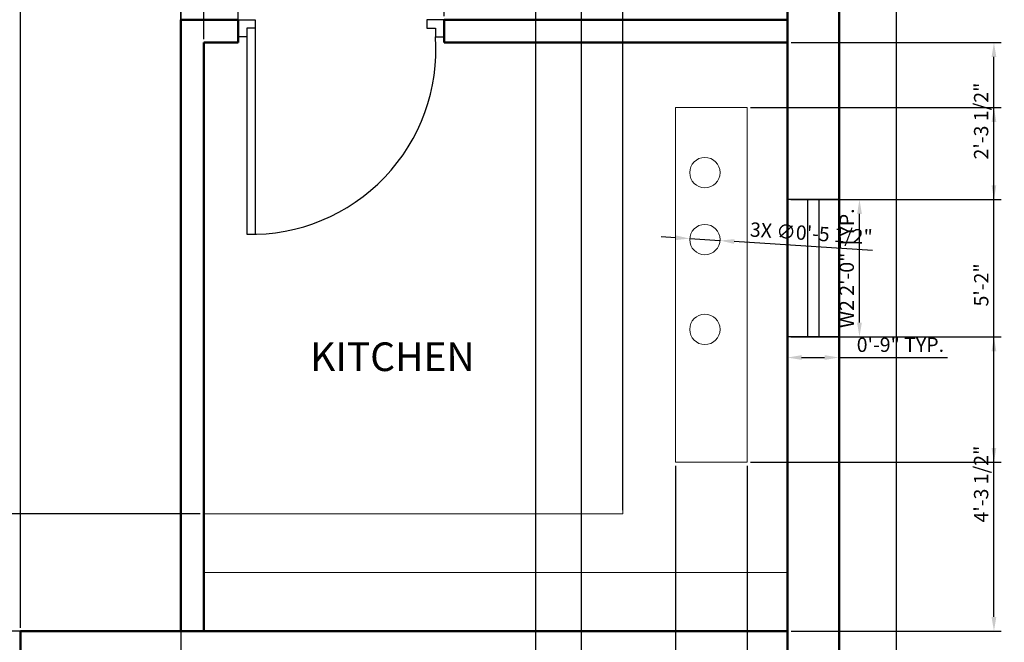
# Model space of a CAD drawing. Units: inches. Extents: x 1905 to 2315, y 3232 to 3824.
# Tile 4 of 8: x 2143 to 2315, y 3371 to 3479. Entities that reach past the tile are written whole.
import ezdxf

# ---------------------------------------------------------------- set-up
doc = ezdxf.new("R2010")
doc.units = ezdxf.units.IN
for name, color, linetype, lineweight in [('A-ANNO-DIMS', 2, 'Continuous', 18), ('A-AREA-IDEN', 7, 'Continuous', 25), ('A-EQPM', 9, 'Continuous', 18), ('A-FLOR-CABT', 8, 'Continuous', 18), ('door', 1, 'Continuous', 25), ('wall', 2, 'Continuous', 50), ('WINDOW', 60, 'Continuous', 25)]:
    doc.layers.add(name, color=color, linetype=linetype, lineweight=lineweight)
doc.styles.get("Standard").update_dxf_attribs({"font": 'arial.ttf'})
doc.dimstyles.new('ISO-25', dxfattribs={"dimtxt": 2.5, "dimasz": 2.5, "dimexe": 1.25, "dimexo": 0.625, "dimtad": 1, "dimdec": 1, "dimlunit": 3, "dimtxsty": 'Standard', "dimcen": 2.5, "dimadec": 0, "dimazin": 0, "dimtfac": 1, "dimtdec": 1, "dimtmove": 0, "dimatfit": 3, "dimfxl": 1, "dimarcsym": 0})

# ---------------------------------------------------------------- blocks, each defined once
blk = doc.blocks.new('*D16')
at = {"layer": 'A-ANNO-DIMS', "color": 0, "lineweight": -2, "transparency": 16777216}
for p, q in [((2286.63, 3793.23), (2297.23, 3793.23)), ((2295.98, 3790.73), (2295.98, 3279.73)), ((2286.63, 3277.23), (2297.23, 3277.23))]:
    blk.add_line(p, q, dxfattribs=at)
at = {"layer": 'A-ANNO-DIMS', "color": 0, "transparency": 16777216}
for points in [[(2295.57, 3790.73), (2296.4, 3790.73), (2295.98, 3793.23)], [(2295.57, 3279.73), (2296.4, 3279.73), (2295.98, 3277.23)]]:
    blk.add_solid(points, dxfattribs=at)
at = {"layer": 'Defpoints', "color": 0, "transparency": 16777216}
for p in [(2286.01, 3793.23), (2286.01, 3277.23), (2295.98, 3277.23)]:
    blk.add_point(p, dxfattribs=at)
at = {"layer": 'A-ANNO-DIMS', "color": 0, "transparency": 16777216, "insert": (2294.08, 3535.23), "char_height": 2.5, "attachment_point": 5, "rotation": 90}
blk.add_mtext("43'", dxfattribs=at)
blk = doc.blocks.new('DOOR-SWING-36IN')
for p, q in [((36.01, 34.5), (0.01, 34.5)), ((34.51, 36), (37.51, 36)), ((34.51, 34.5), (34.51, 36)), ((36.01, 34.5), (34.51, 34.5)), ((36.01, 33), (36.01, 34.5)), ((37.51, 36), (37.51, 33)), ((36.01, 33), (0.01, 33)), ((37.51, 33), (36.01, 33)), ((37.51, 3), (36.01, 3)), ((36.01, 3), (36.01, 1.5)), ((37.51, 0), (37.51, 3)), ((36.01, 1.5), (34.51, 1.5)), ((34.51, 1.5), (34.51, 0)), ((34.51, 0), (37.51, 0))]:
    blk.add_line(p, q)
blk.add_arc((32.32, 33.75), 32.32, 178.6705, 273.8756)
blk = doc.blocks.new('WIN-24IN')
for p, q in [((9, 24), (0, 24)), ((0, 24), (0, 0)), ((3.5, 24), (3.5, 0)), ((5.5, 24), (5.5, 0)), ((9, 24), (9, 0)), ((9, 0), (0, 0))]:
    blk.add_line(p, q)
blk = doc.blocks.new('*D23')
at = {"layer": 'A-ANNO-DIMS', "color": 0, "lineweight": -2, "transparency": 16777216}
for p, q in [((2286.6, 3448.02), (2290.82, 3448.02)), ((2289.57, 3426.52), (2289.57, 3445.52)), ((2286.6, 3424.02), (2290.82, 3424.02))]:
    blk.add_line(p, q, dxfattribs=at)
at = {"layer": 'A-ANNO-DIMS', "color": 0, "transparency": 16777216}
for points in [[(2289.16, 3445.52), (2289.99, 3445.52), (2289.57, 3448.02)], [(2289.16, 3426.52), (2289.99, 3426.52), (2289.57, 3424.02)]]:
    blk.add_solid(points, dxfattribs=at)
at = {"layer": 'Defpoints', "color": 0, "transparency": 16777216}
for p in [(2285.97, 3448.02), (2289.57, 3448.02), (2285.97, 3424.02)]:
    blk.add_point(p, dxfattribs=at)
at = {"layer": 'A-ANNO-DIMS', "color": 0, "transparency": 16777216, "insert": (2287.67, 3436.02), "char_height": 2.5, "attachment_point": 5, "rotation": 90}
blk.add_mtext('W2 2\'-0" TYP.', dxfattribs=at)
blk = doc.blocks.new('*D24')
at = {"layer": 'A-ANNO-DIMS', "color": 0, "lineweight": -2, "transparency": 16777216}
for p, q in [((2276.97, 3423.4), (2276.97, 3419.17)), ((2285.97, 3423.4), (2285.97, 3419.17)), ((2279.47, 3420.42), (2283.47, 3420.42)), ((2285.97, 3420.42), (2304.96, 3420.42))]:
    blk.add_line(p, q, dxfattribs=at)
at = {"layer": 'A-ANNO-DIMS', "color": 0, "transparency": 16777216}
for points in [[(2279.47, 3420.84), (2279.47, 3420.01), (2276.97, 3420.42)], [(2283.47, 3420.84), (2283.47, 3420.01), (2285.97, 3420.42)]]:
    blk.add_solid(points, dxfattribs=at)
at = {"layer": 'Defpoints', "color": 0, "transparency": 16777216}
for p in [(2276.97, 3424.02), (2285.97, 3424.02), (2285.97, 3420.42)]:
    blk.add_point(p, dxfattribs=at)
at = {"layer": 'A-ANNO-DIMS', "color": 0, "transparency": 16777216, "insert": (2296.72, 3422.33), "char_height": 2.5, "attachment_point": 5}
blk.add_mtext('0\'-9" TYP.', dxfattribs=at)
blk = doc.blocks.new('*D41')
at = {"layer": 'A-ANNO-DIMS', "color": 0, "lineweight": -2, "transparency": 16777216}
for p, q in [((2095.01, 3663.61), (2095.01, 3232.16)), ((2171.01, 3663.61), (2171.01, 3232.16)), ((2097.51, 3233.41), (2168.51, 3233.41))]:
    blk.add_line(p, q, dxfattribs=at)
at = {"layer": 'A-ANNO-DIMS', "color": 0, "transparency": 16777216}
for points in [[(2097.51, 3233.83), (2097.51, 3233), (2095.01, 3233.41)], [(2168.51, 3233.83), (2168.51, 3233), (2171.01, 3233.41)]]:
    blk.add_solid(points, dxfattribs=at)
at = {"layer": 'Defpoints', "color": 0, "transparency": 16777216}
for p in [(2095.01, 3664.23), (2171.01, 3664.23), (2171.01, 3233.41)]:
    blk.add_point(p, dxfattribs=at)
at = {"layer": 'A-ANNO-DIMS', "color": 0, "transparency": 16777216, "insert": (2133.01, 3235.31), "char_height": 2.5, "attachment_point": 5}
blk.add_mtext('6\'-4"', dxfattribs=at)
blk = doc.blocks.new('*D51')
at = {"layer": 'A-ANNO-DIMS', "color": 0, "lineweight": -2, "transparency": 16777216}
for p, q in [((2277.6, 3424.02), (2314.32, 3424.02)), ((2313.07, 3375.1), (2313.07, 3421.52)), ((2277.63, 3372.6), (2314.32, 3372.6))]:
    blk.add_line(p, q, dxfattribs=at)
at = {"layer": 'A-ANNO-DIMS', "color": 0, "transparency": 16777216}
for points in [[(2312.65, 3421.52), (2313.48, 3421.52), (2313.07, 3424.02)], [(2312.65, 3375.1), (2313.48, 3375.1), (2313.07, 3372.6)]]:
    blk.add_solid(points, dxfattribs=at)
at = {"layer": 'Defpoints', "color": 0, "transparency": 16777216}
for p in [(2276.97, 3424.02), (2313.07, 3424.02), (2277.01, 3372.6)]:
    blk.add_point(p, dxfattribs=at)
at = {"layer": 'A-ANNO-DIMS', "color": 0, "transparency": 16777216, "insert": (2311.15, 3398.31), "char_height": 2.5, "attachment_point": 5, "rotation": 90}
blk.add_mtext('4\'-3 1/2"', dxfattribs=at)
blk = doc.blocks.new('*D52')
at = {"layer": 'A-ANNO-DIMS', "color": 0, "lineweight": -2, "transparency": 16777216}
for p, q in [((2277.63, 3475.45), (2314.32, 3475.45)), ((2313.07, 3450.52), (2313.07, 3472.95)), ((2277.6, 3448.02), (2314.32, 3448.02))]:
    blk.add_line(p, q, dxfattribs=at)
at = {"layer": 'A-ANNO-DIMS', "color": 0, "transparency": 16777216}
for points in [[(2312.65, 3472.95), (2313.48, 3472.95), (2313.07, 3475.45)], [(2312.65, 3450.52), (2313.48, 3450.52), (2313.07, 3448.02)]]:
    blk.add_solid(points, dxfattribs=at)
at = {"layer": 'Defpoints', "color": 0, "transparency": 16777216}
for p in [(2277.01, 3475.45), (2313.07, 3475.45), (2276.97, 3448.02)]:
    blk.add_point(p, dxfattribs=at)
at = {"layer": 'A-ANNO-DIMS', "color": 0, "transparency": 16777216, "insert": (2311.15, 3461.74), "char_height": 2.5, "attachment_point": 5, "rotation": 90}
blk.add_mtext('2\'-3 1/2"', dxfattribs=at)
blk = doc.blocks.new('*D62')
at = {"layer": 'A-ANNO-DIMS', "color": 0, "lineweight": -2, "transparency": 16777216}
for p, q in [((2233.01, 3322.86), (2233.01, 3821.54)), ((2241.01, 3322.86), (2241.01, 3821.54)), ((2235.51, 3820.29), (2238.51, 3820.29))]:
    blk.add_line(p, q, dxfattribs=at)
at = {"layer": 'A-ANNO-DIMS', "color": 0, "transparency": 16777216}
for points in [[(2235.51, 3820.71), (2235.51, 3819.88), (2233.01, 3820.29)], [(2238.51, 3820.71), (2238.51, 3819.88), (2241.01, 3820.29)]]:
    blk.add_solid(points, dxfattribs=at)
at = {"layer": 'Defpoints', "color": 0, "transparency": 16777216}
for p in [(2241.01, 3820.29), (2233.01, 3322.23), (2241.01, 3322.23)]:
    blk.add_point(p, dxfattribs=at)
at = {"layer": 'A-ANNO-DIMS', "color": 0, "transparency": 16777216, "insert": (2237.01, 3822.19), "char_height": 2.5, "attachment_point": 5}
blk.add_mtext('0\'-8"', dxfattribs=at)
blk = doc.blocks.new('*D63')
at = {"layer": 'A-ANNO-DIMS', "color": 0, "lineweight": -2, "transparency": 16777216}
for p, q in [((2171.01, 3480.07), (2171.01, 3821.54)), ((2175.01, 3476.07), (2175.01, 3821.54)), ((2168.51, 3820.29), (2166.01, 3820.29)), ((2171.01, 3820.29), (2175.01, 3820.29)), ((2177.51, 3820.29), (2187.9, 3820.29))]:
    blk.add_line(p, q, dxfattribs=at)
at = {"layer": 'A-ANNO-DIMS', "color": 0, "transparency": 16777216}
for points in [[(2168.51, 3820.71), (2168.51, 3819.88), (2171.01, 3820.29)], [(2177.51, 3820.71), (2177.51, 3819.88), (2175.01, 3820.29)]]:
    blk.add_solid(points, dxfattribs=at)
at = {"layer": 'Defpoints', "color": 0, "transparency": 16777216}
for p in [(2175.01, 3820.29), (2171.01, 3479.45), (2175.01, 3475.45)]:
    blk.add_point(p, dxfattribs=at)
at = {"layer": 'A-ANNO-DIMS', "color": 0, "transparency": 16777216, "insert": (2183.96, 3822.19), "char_height": 2.5, "attachment_point": 5}
blk.add_mtext('0\'-4"', dxfattribs=at)
blk = doc.blocks.new('*D66')
at = {"layer": 'A-ANNO-DIMS', "color": 0, "lineweight": -2, "transparency": 16777216}
for p, q in [((2248.2, 3393.73), (2248.2, 3821.54)), ((2277.01, 3383.48), (2277.01, 3821.54)), ((2250.7, 3820.29), (2274.51, 3820.29))]:
    blk.add_line(p, q, dxfattribs=at)
at = {"layer": 'A-ANNO-DIMS', "color": 0, "transparency": 16777216}
for points in [[(2250.7, 3820.71), (2250.7, 3819.88), (2248.2, 3820.29)], [(2274.51, 3820.71), (2274.51, 3819.88), (2277.01, 3820.29)]]:
    blk.add_solid(points, dxfattribs=at)
at = {"layer": 'Defpoints', "color": 0, "transparency": 16777216}
for p in [(2277.01, 3820.29), (2248.2, 3393.11), (2277.01, 3382.85)]:
    blk.add_point(p, dxfattribs=at)
at = {"layer": 'A-ANNO-DIMS', "color": 0, "transparency": 16777216, "insert": (2262.6, 3822.19), "char_height": 2.5, "attachment_point": 5}
blk.add_mtext('2\'-5"', dxfattribs=at)
blk = doc.blocks.new('*D67')
at = {"layer": 'A-ANNO-DIMS', "color": 0, "lineweight": -2, "transparency": 16777216}
for p, q in [((2174.38, 3393.11), (1909.7, 3393.11)), ((1910.95, 3375.1), (1910.95, 3390.61)), ((2174.38, 3372.6), (1909.7, 3372.6))]:
    blk.add_line(p, q, dxfattribs=at)
at = {"layer": 'A-ANNO-DIMS', "color": 0, "transparency": 16777216}
for points in [[(1910.53, 3390.61), (1911.36, 3390.61), (1910.95, 3393.11)], [(1910.53, 3375.1), (1911.36, 3375.1), (1910.95, 3372.6)]]:
    blk.add_solid(points, dxfattribs=at)
at = {"layer": 'Defpoints', "color": 0, "transparency": 16777216}
for p in [(1910.95, 3393.11), (2175.01, 3393.11), (2175.01, 3372.6)]:
    blk.add_point(p, dxfattribs=at)
at = {"layer": 'A-ANNO-DIMS', "color": 0, "transparency": 16777216, "insert": (1909.03, 3382.85), "char_height": 2.5, "attachment_point": 5, "rotation": 90}
blk.add_mtext('1\'-8 1/2"', dxfattribs=at)
blk = doc.blocks.new('*D68')
at = {"layer": 'A-ANNO-DIMS', "color": 0, "lineweight": -2, "transparency": 16777216}
for p, q in [((2257.4, 3401.51), (2257.4, 3232.16)), ((2269.93, 3401.51), (2269.93, 3232.16)), ((2259.9, 3233.41), (2267.43, 3233.41)), ((2269.93, 3233.41), (2285.92, 3233.41))]:
    blk.add_line(p, q, dxfattribs=at)
at = {"layer": 'A-ANNO-DIMS', "color": 0, "transparency": 16777216}
for points in [[(2259.9, 3233.83), (2259.9, 3233), (2257.4, 3233.41)], [(2267.43, 3233.83), (2267.43, 3233), (2269.93, 3233.41)]]:
    blk.add_solid(points, dxfattribs=at)
at = {"layer": 'Defpoints', "color": 0, "transparency": 16777216}
for p in [(2257.4, 3402.13), (2269.93, 3402.13), (2269.93, 3233.41)]:
    blk.add_point(p, dxfattribs=at)
at = {"layer": 'A-ANNO-DIMS', "color": 0, "transparency": 16777216, "insert": (2279.17, 3235.33), "char_height": 2.5, "attachment_point": 5}
blk.add_mtext('1\'-0 1/2"', dxfattribs=at)
blk = doc.blocks.new('*D69')
at = {"layer": 'A-ANNO-DIMS', "color": 0, "lineweight": -2, "transparency": 16777216}
for p, q in [((2270.56, 3464.09), (2314.32, 3464.09)), ((2313.07, 3404.63), (2313.07, 3461.59)), ((2270.56, 3402.13), (2314.32, 3402.13))]:
    blk.add_line(p, q, dxfattribs=at)
at = {"layer": 'A-ANNO-DIMS', "color": 0, "transparency": 16777216}
for points in [[(2312.65, 3461.59), (2313.48, 3461.59), (2313.07, 3464.09)], [(2312.65, 3404.63), (2313.48, 3404.63), (2313.07, 3402.13)]]:
    blk.add_solid(points, dxfattribs=at)
at = {"layer": 'Defpoints', "color": 0, "transparency": 16777216}
for p in [(2269.93, 3464.09), (2313.07, 3464.09), (2269.93, 3402.13)]:
    blk.add_point(p, dxfattribs=at)
at = {"layer": 'A-ANNO-DIMS', "color": 0, "transparency": 16777216, "insert": (2311.17, 3433.11), "char_height": 2.5, "attachment_point": 5, "rotation": 90}
blk.add_mtext('5\'-2"', dxfattribs=at)
blk = doc.blocks.new('*D70')
at = {"layer": 'A-ANNO-DIMS', "color": 0, "lineweight": -2, "transparency": 16777216}
for p, q in [((2175.01, 3476.07), (2175.01, 3821.54)), ((2181.01, 3476.07), (2181.01, 3821.54)), ((2172.51, 3820.29), (2170.01, 3820.29)), ((2175.01, 3820.29), (2181.01, 3820.29)), ((2183.51, 3820.29), (2193.9, 3820.29))]:
    blk.add_line(p, q, dxfattribs=at)
at = {"layer": 'A-ANNO-DIMS', "color": 0, "transparency": 16777216}
for points in [[(2172.51, 3820.71), (2172.51, 3819.88), (2175.01, 3820.29)], [(2183.51, 3820.71), (2183.51, 3819.88), (2181.01, 3820.29)]]:
    blk.add_solid(points, dxfattribs=at)
at = {"layer": 'Defpoints', "color": 0, "transparency": 16777216}
for p in [(2181.01, 3820.29), (2175.01, 3475.45), (2181.01, 3475.45)]:
    blk.add_point(p, dxfattribs=at)
at = {"layer": 'A-ANNO-DIMS', "color": 0, "transparency": 16777216, "insert": (2189.96, 3822.19), "char_height": 2.5, "attachment_point": 5}
blk.add_mtext('0\'-6"', dxfattribs=at)
blk = doc.blocks.new('*D71')
at = {"layer": 'A-ANNO-DIMS', "color": 0, "lineweight": -2, "transparency": 16777216}
for p, q in [((2217.01, 3480.07), (2217.01, 3821.54)), ((2277.01, 3476.07), (2277.01, 3821.54)), ((2219.51, 3820.29), (2274.51, 3820.29))]:
    blk.add_line(p, q, dxfattribs=at)
at = {"layer": 'A-ANNO-DIMS', "color": 0, "transparency": 16777216}
for points in [[(2219.51, 3820.71), (2219.51, 3819.88), (2217.01, 3820.29)], [(2274.51, 3820.71), (2274.51, 3819.88), (2277.01, 3820.29)]]:
    blk.add_solid(points, dxfattribs=at)
at = {"layer": 'Defpoints', "color": 0, "transparency": 16777216}
for p in [(2277.01, 3820.29), (2217.01, 3479.45), (2277.01, 3475.45)]:
    blk.add_point(p, dxfattribs=at)
at = {"layer": 'A-ANNO-DIMS', "color": 0, "transparency": 16777216, "insert": (2247.01, 3822.19), "char_height": 2.5, "attachment_point": 5}
blk.add_mtext('5\'-0"', dxfattribs=at)
blk = doc.blocks.new('*D72')
at = {"layer": 'A-ANNO-DIMS', "color": 0, "lineweight": -2, "transparency": 16777216}
for p, q in [((2143.01, 3373.22), (2143.01, 3821.54)), ((2171.01, 3373.22), (2171.01, 3821.54)), ((2145.51, 3820.29), (2168.51, 3820.29))]:
    blk.add_line(p, q, dxfattribs=at)
at = {"layer": 'A-ANNO-DIMS', "color": 0, "transparency": 16777216}
for points in [[(2145.51, 3820.71), (2145.51, 3819.88), (2143.01, 3820.29)], [(2168.51, 3820.71), (2168.51, 3819.88), (2171.01, 3820.29)]]:
    blk.add_solid(points, dxfattribs=at)
at = {"layer": 'Defpoints', "color": 0, "transparency": 16777216}
for p in [(2171.01, 3820.29), (2143.01, 3372.6), (2171.01, 3372.6)]:
    blk.add_point(p, dxfattribs=at)
at = {"layer": 'A-ANNO-DIMS', "color": 0, "transparency": 16777216, "insert": (2157.01, 3822.17), "char_height": 2.5, "attachment_point": 5}
blk.add_mtext('2\'-4"', dxfattribs=at)
blk = doc.blocks.new('*D76')
at = {"layer": 'A-ANNO-DIMS', "color": 0, "lineweight": -2, "transparency": 16777216}
for p, q in [((2257.42, 3441.36), (2254.93, 3441.52)), ((2259.92, 3441.2), (2265.2, 3440.86)), ((2291.82, 3439.15), (2267.69, 3440.7))]:
    blk.add_line(p, q, dxfattribs=at)
at = {"layer": 'A-ANNO-DIMS', "color": 0, "transparency": 16777216}
for points in [[(2257.45, 3441.77), (2257.4, 3440.94), (2259.92, 3441.2)], [(2267.72, 3441.11), (2267.67, 3440.28), (2265.2, 3440.86)]]:
    blk.add_solid(points, dxfattribs=at)
at = {"layer": 'Defpoints', "color": 0, "transparency": 16777216}
for p in [(2259.92, 3441.2), (2265.2, 3440.86)]:
    blk.add_point(p, dxfattribs=at)
at = {"layer": 'A-ANNO-DIMS', "color": 0, "transparency": 16777216, "insert": (2281.13, 3441.81), "char_height": 2.5, "attachment_point": 5, "rotation": 356.3377}
blk.add_mtext('3X ∅0\'-5 1/2"', dxfattribs=at)

msp = doc.modelspace()

# ---------------------------------------------------------------- linework, layer by layer
at = {"layer": 'A-EQPM'}
msp.add_lwpolyline([(2257.4, 3464.09), (2269.93, 3464.09), (2269.93, 3402.13), (2257.4, 3402.13)], close=True, dxfattribs=at)
for centre in [(2262.56, 3452.73), (2262.56, 3441.03), (2262.56, 3425.34)]:
    msp.add_circle(centre, 2.65, dxfattribs=at)
at = {"layer": 'A-FLOR-CABT'}
for p, q in [((2277.01, 3475.45), (2248.2, 3475.45)), ((2248.2, 3475.45), (2248.2, 3393.11)), ((2277.01, 3372.6), (2277.01, 3475.45)), ((2248.2, 3393.11), (2175.01, 3393.11)), ((2175.01, 3393.11), (2175.01, 3372.6)), ((2277.01, 3372.6), (2277.01, 3393.11)), ((2175.01, 3372.6), (2277.01, 3372.6)), ((2248.2, 3372.6), (2277.01, 3372.6))]:
    msp.add_line(p, q, dxfattribs=at)
msp.add_lwpolyline([(2175.01, 3382.85), (2277.01, 3382.85), (2277.01, 3382.85), (2175.01, 3382.85)], close=True, dxfattribs=at)
at = {"layer": 'wall'}
for p, q in [((2286.01, 3277.23), (2286.01, 3793.23)), ((2277.01, 3286.23), (2277.01, 3784.23)), ((2171.01, 3372.6), (2171.01, 3479.45)), ((2181.01, 3479.45), (2171.01, 3479.45)), ((2181.01, 3475.45), (2181.01, 3479.45)), ((2277.01, 3479.45), (2217.01, 3479.45)), ((2217.01, 3475.45), (2217.01, 3479.45)), ((2175.01, 3372.6), (2175.01, 3475.45)), ((2181.01, 3475.45), (2175.01, 3475.45)), ((2277.01, 3475.45), (2217.01, 3475.45)), ((2277.01, 3372.6), (2143.01, 3372.6)), ((2143.01, 3372.6), (2143.01, 3368.6))]:
    msp.add_line(p, q, dxfattribs=at)

# ---------------------------------------------------------------- block references
at = {"layer": 'door', "rotation": 90.00000000000367}
msp.add_blockref('DOOR-SWING-36IN', (2217.01, 3441.94), dxfattribs=at)
at = {"layer": 'WINDOW'}
msp.add_blockref('WIN-24IN', (2276.97, 3424.03), dxfattribs=at)

# ---------------------------------------------------------------- texts
at = {"layer": 'A-AREA-IDEN', "insert": (2193.59, 3423.06), "char_height": 5, "attachment_point": 1}
msp.add_mtext_dynamic_manual_height_columns('KITCHEN', width=56.1502, gutter_width=12.5, heights=[0], dxfattribs=at)

# ---------------------------------------------------------------- dimensions: what is measured, and where the dimension line sits
at = {"layer": 'A-ANNO-DIMS'}
for base, p1, p2, picture, middle in [((2171.01, 3820.29), (2143.01, 3372.6), (2171.01, 3372.6), '*D72', (2157.01, 3822.17)), ((2175.01, 3820.29), (2171.01, 3479.45), (2175.01, 3475.45), '*D63', (2183.96, 3822.19)), ((2181.01, 3820.29), (2175.01, 3475.45), (2181.01, 3475.45), '*D70', (2189.96, 3822.19)), ((2277.01, 3820.29), (2217.01, 3479.45), (2277.01, 3475.45), '*D71', (2247.01, 3822.19)), ((2241.01, 3820.29), (2233.01, 3322.23), (2241.01, 3322.23), '*D62', (2237.01, 3822.19)), ((2277.01, 3820.29), (2248.2, 3393.11), (2277.01, 3382.85), '*D66', (2262.6, 3822.19)), ((2171.01, 3233.41), (2095.01, 3664.23), (2171.01, 3664.23), '*D41', (2133.01, 3235.31)), ((2269.93, 3233.41), (2257.4, 3402.13), (2269.93, 3402.13), '*D68', (2279.17, 3235.33))]:
    dim = msp.add_linear_dim(base=base, p1=p1, p2=p2, dimstyle='ISO-25', override={"dimdec": 1, "dimlfac": 1, "dimrnd": 0, "dimzin": 1, "dimdsep": 46, "dimlunit": 4, "dimfrac": 2}, dxfattribs=at)
    dim.commit()
    dim.dimension.update_dxf_attribs({"geometry": picture, "text_midpoint": middle})
for base, p1, p2, override, picture, middle in [((2295.98, 3277.23), (2286.01, 3793.23), (2286.01, 3277.23), {"dimclrd": 0, "dimclre": 0, "dimclrt": 0}, '*D16', (2294.08, 3535.23)), ((2313.07, 3475.45), (2276.97, 3448.02), (2277.01, 3475.45), {"dimdec": 1, "dimlfac": 1, "dimrnd": 0, "dimzin": 1, "dimdsep": 46, "dimlunit": 4, "dimfrac": 2}, '*D52', (2311.15, 3461.74)), ((2313.07, 3464.09), (2269.93, 3402.13), (2269.93, 3464.09), {"dimdec": 1, "dimlfac": 1, "dimrnd": 0, "dimzin": 1, "dimdsep": 46, "dimlunit": 4, "dimfrac": 2}, '*D69', (2311.17, 3433.11)), ((2313.07, 3424.02), (2277.01, 3372.6), (2276.97, 3424.02), {"dimdec": 1, "dimlfac": 1, "dimrnd": 0, "dimzin": 1, "dimdsep": 46, "dimlunit": 4, "dimfrac": 2}, '*D51', (2311.15, 3398.31)), ((1910.95, 3393.11), (2175.01, 3372.6), (2175.01, 3393.11), {"dimdec": 1, "dimlfac": 1, "dimrnd": 0, "dimzin": 1, "dimdsep": 46, "dimlunit": 4, "dimfrac": 2}, '*D67', (1909.03, 3382.85))]:
    dim = msp.add_linear_dim(base=base, p1=p1, p2=p2, angle=90, dimstyle='ISO-25', override=override, dxfattribs=at)
    dim.commit()
    dim.dimension.update_dxf_attribs({"geometry": picture, "text_midpoint": middle})
dim = msp.add_diameter_dim_2p(p1=(2259.92, 3441.2), p2=(2265.2, 3440.86), text='3X <>', dimstyle='ISO-25', override={"dimdec": 1, "dimlfac": 1, "dimrnd": 0, "dimzin": 1, "dimdsep": 46, "dimlunit": 4, "dimfrac": 2}, dxfattribs=at)
dim.commit()
dim.dimension.update_dxf_attribs({"geometry": '*D76', "text_midpoint": (2281, 3439.85)})
dim = msp.add_linear_dim(base=(2289.57, 3448.02), p1=(2285.97, 3424.02), p2=(2285.97, 3448.02), angle=90, text='W2 <> TYP.', dimstyle='ISO-25', override={"dimdec": 1, "dimlfac": 1, "dimrnd": 0, "dimzin": 1, "dimdsep": 46, "dimlunit": 4, "dimfrac": 2}, dxfattribs=at)
dim.commit()
dim.dimension.update_dxf_attribs({"geometry": '*D23', "text_midpoint": (2287.67, 3436.02)})
dim = msp.add_linear_dim(base=(2285.97, 3420.42), p1=(2276.97, 3424.02), p2=(2285.97, 3424.02), text='<> TYP.', dimstyle='ISO-25', override={"dimdec": 1, "dimlfac": 1, "dimrnd": 0, "dimzin": 1, "dimdsep": 46, "dimlunit": 4, "dimfrac": 2}, dxfattribs=at)
dim.commit()
dim.dimension.update_dxf_attribs({"geometry": '*D24', "text_midpoint": (2296.72, 3422.33)})

doc.saveas('drawing.dxf')
